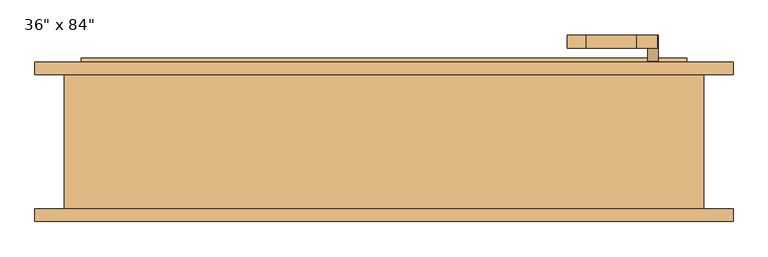
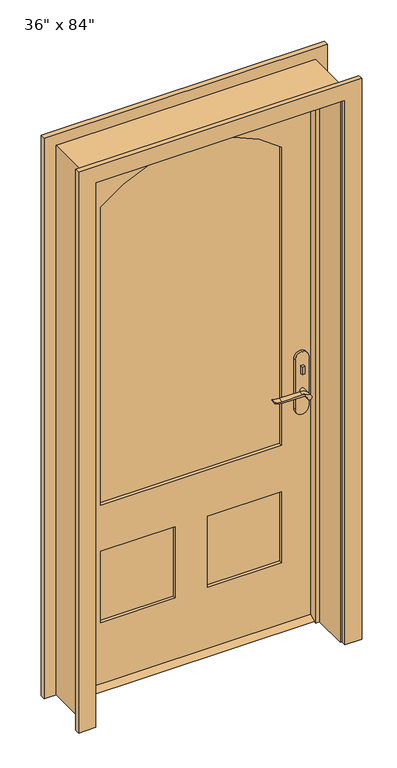
"""IFC4 building model written with IfcOpenShell, lengths in millimetres: door geometry."""

from ifc_helpers import new_model, si_unit, point, frame, frame_2d, origin, place, context, project, spatial, polyline, circle_curve, trimmed, segment, composite_curve, outline, extrude, faceted_brep, source, transform, mapped, element, save


def door_4a215221(model_context):
    return source(origin(), model_context, "Body", "SolidModel", [
        extrude(outline(polyline([(63.5, 12.7), (98.425, 12.7), (123.825, 0.0), (38.1, 0.0), (63.5, 12.7)])), frame((-457.2, 0.0, 0.0), z_axis=(1.0, 0.0, 0.0), x_axis=(0.0, 1.0, 0.0)), (0.0, 0.0, 1.0), 914.4),
        extrude(outline(polyline([(411.4, 43.5), (401.4, 43.5), (401.4, 53.5), (411.4, 53.5), (411.4, 43.5)])), frame((0.0, 0.0, 981.9), z_axis=(0.0, 0.0, 1.0), x_axis=(1.0, 0.0, 0.0)), (0.0, 0.0, 1.0), 30.0),
        extrude(outline(composite_curve([segment(trimmed(circle_curve(frame_2d((996.9, 406.4)), 8.0), [point((996.9, 398.4))], [point((996.9, 414.4))], False, "CARTESIAN"), True, "CONTINUOUS"), segment(trimmed(circle_curve(frame_2d((996.9, 406.4)), 8.0), [point((996.9, 414.4))], [point((996.9, 398.4))], False, "CARTESIAN"), True, "CONTINUOUS")], self_intersect=False)), frame((0.0, 108.425, 0.0), z_axis=(0.0, 1.0, 0.0), x_axis=(0.0, 0.0, 1.0)), (0.0, 0.0, 1.0), 10.0),
        extrude(outline(composite_curve([segment(trimmed(circle_curve(frame_2d((897.1555521, 382.7324871)), 37.2832219), [point((919.0523287, 412.9081363))], [point((934.4, 381.0325667))], False, "CARTESIAN"), True, "CONTINUOUS"), segment(polyline([(934.4, 381.0325667), (934.4, 304.7564091)]), True, "CONTINUOUS"), segment(trimmed(circle_curve(frame_2d((1017.6850638, 304.8227909)), 83.2850902), [point((934.4, 304.7564091))], [point((939.4, 276.4))], True, "CARTESIAN"), True, "CONTINUOUS"), segment(polyline([(939.4, 276.4), (936.6135558, 276.4)]), True, "CONTINUOUS"), segment(trimmed(circle_curve(frame_2d((986.6709207, 308.3396612)), 59.3791355), [point((936.6135558, 276.4))], [point((927.4, 304.7564091))], False, "CARTESIAN"), True, "CONTINUOUS"), segment(polyline([(927.4, 304.7564091), (927.4, 381.0138099)]), True, "CONTINUOUS"), segment(trimmed(circle_curve(frame_2d((909.2738613, 381.0138099)), 18.1261387), [point((927.4, 381.0138099))], [point((914.4, 398.4))], True, "CARTESIAN"), True, "CONTINUOUS"), segment(trimmed(circle_curve(frame_2d((914.4, 406.4)), 8.0), [point((914.4, 398.4))], [point((919.0523287, 412.9081363))], False, "CARTESIAN"), True, "CONTINUOUS")], self_intersect=False)), frame((0.0, 3.5, 0.0), z_axis=(0.0, 1.0, 0.0), x_axis=(0.0, 0.0, 1.0)), (0.0, 0.0, 1.0), 20.0),
        extrude(outline(composite_curve([segment(trimmed(circle_curve(frame_2d((914.4, 406.4)), 8.0), [point((914.3999903, 398.4))], [point((919.0523287, 412.9081363))], False, "CARTESIAN"), True, "CONTINUOUS"), segment(trimmed(circle_curve(frame_2d((897.1555521, 382.7324871)), 37.2832219), [point((919.0523287, 412.9081363))], [point((934.4, 381.0325667))], False, "CARTESIAN"), True, "CONTINUOUS"), segment(polyline([(934.4, 381.0325667), (934.4, 304.7564091)]), True, "CONTINUOUS"), segment(trimmed(circle_curve(frame_2d((1017.6850638, 304.8227909)), 83.2850902), [point((934.4, 304.7564091))], [point((939.4, 276.4))], True, "CARTESIAN"), True, "CONTINUOUS"), segment(polyline([(939.4, 276.4), (936.6135558, 276.4)]), True, "CONTINUOUS"), segment(trimmed(circle_curve(frame_2d((986.6709207, 308.3396612)), 59.3791355), [point((936.6135558, 276.4))], [point((927.4, 304.7564091))], False, "CARTESIAN"), True, "CONTINUOUS"), segment(polyline([(927.4, 304.7564091), (927.4, 381.0138122)]), True, "CONTINUOUS"), segment(trimmed(circle_curve(frame_2d((909.2738682, 381.0138122)), 18.1261318), [point((927.4, 381.0138122))], [point((914.3999903, 398.4))], True, "CARTESIAN"), True, "CONTINUOUS")], self_intersect=False)), frame((0.0, 138.425, 0.0), z_axis=(0.0, 1.0, 0.0), x_axis=(0.0, 0.0, 1.0)), (0.0, 0.0, 1.0), 20.0),
        extrude(outline(composite_curve([segment(trimmed(circle_curve(frame_2d((914.4, 406.4)), 8.0), [point((914.4, 398.4))], [point((914.4, 414.4))], False, "CARTESIAN"), True, "CONTINUOUS"), segment(trimmed(circle_curve(frame_2d((914.4, 406.4)), 8.0), [point((914.4, 414.4))], [point((914.4, 398.4))], False, "CARTESIAN"), True, "CONTINUOUS")], self_intersect=False)), frame((0.0, 23.5, 0.0), z_axis=(0.0, 1.0, 0.0), x_axis=(0.0, 0.0, 1.0)), (0.0, 0.0, 1.0), 30.0),
        extrude(outline(composite_curve([segment(trimmed(circle_curve(frame_2d((914.4, 406.4)), 8.0), [point((914.4, 398.4))], [point((914.4, 414.4))], False, "CARTESIAN"), True, "CONTINUOUS"), segment(trimmed(circle_curve(frame_2d((914.4, 406.4)), 8.0), [point((914.4, 414.4))], [point((914.4, 398.4))], False, "CARTESIAN"), True, "CONTINUOUS")], self_intersect=False)), frame((0.0, 108.425, 0.0), z_axis=(0.0, 1.0, 0.0), x_axis=(0.0, 0.0, 1.0)), (0.0, 0.0, 1.0), 30.0),
        extrude(outline(composite_curve([segment(polyline([(844.4, 431.4), (1039.4, 431.4)]), True, "CONTINUOUS"), segment(trimmed(circle_curve(frame_2d((1039.4, 406.4)), 25.0), [point((1039.4, 431.4))], [point((1039.4, 381.4))], False, "CARTESIAN"), True, "CONTINUOUS"), segment(polyline([(1039.4, 381.4), (844.4, 381.4)]), True, "CONTINUOUS"), segment(trimmed(circle_curve(frame_2d((844.4, 406.4)), 25.0), [point((844.4, 381.4))], [point((844.4, 431.4))], False, "CARTESIAN"), True, "CONTINUOUS")], self_intersect=False)), frame((0.0, 53.5, 0.0), z_axis=(0.0, 1.0, 0.0), x_axis=(0.0, 0.0, 1.0)), (0.0, 0.0, 1.0), 10.0),
        extrude(outline(composite_curve([segment(polyline([(844.4, 431.4), (1039.4, 431.4)]), True, "CONTINUOUS"), segment(trimmed(circle_curve(frame_2d((1039.4, 406.4)), 25.0), [point((1039.4, 431.4))], [point((1039.4, 381.4))], False, "CARTESIAN"), True, "CONTINUOUS"), segment(polyline([(1039.4, 381.4), (844.4, 381.4)]), True, "CONTINUOUS"), segment(trimmed(circle_curve(frame_2d((844.4, 406.4)), 25.0), [point((844.4, 381.4))], [point((844.4, 431.4))], False, "CARTESIAN"), True, "CONTINUOUS")], self_intersect=False)), frame((0.0, 98.425, 0.0), z_axis=(0.0, 1.0, 0.0), x_axis=(0.0, 0.0, 1.0)), (0.0, 0.0, 1.0), 10.0),
        extrude(outline(polyline([(2133.6, -457.2), (12.7, -457.2), (12.7, 457.2), (2133.6, 457.2), (2133.6, -457.2)]), holes=[composite_curve([segment(polyline([(714.375, -336.55), (1885.95, -336.55)]), True, "CONTINUOUS"), segment(trimmed(circle_curve(frame_2d((1503.52125, 0.0)), 509.42875), [point((1885.95, -336.55))], [point((1885.95, 336.55))], True, "CARTESIAN"), True, "CONTINUOUS"), segment(polyline([(1885.95, 336.55), (714.375, 336.55), (714.375, -336.55)]), True, "CONTINUOUS")], self_intersect=False), polyline([(533.4, -60.325), (254.0, -60.325), (254.0, -336.55), (533.4, -336.55), (533.4, -60.325)]), polyline([(533.4, 336.55), (254.0, 336.55), (254.0, 60.325), (533.4, 60.325), (533.4, 336.55)])]), frame((0.0, 63.5, 0.0), z_axis=(0.0, 1.0, 0.0), x_axis=(0.0, 0.0, 1.0)), (0.0, 0.0, 1.0), 34.925),
        faceted_brep([(482.6, 98.425, 0.0), (482.6, -104.775, 0.0), (457.2, -104.775, 0.0), (457.2, 28.575, 0.0), (444.5, 28.575, 0.0), (444.5, 63.5, 0.0), (457.2, 63.5, 0.0), (457.2, 98.425, 0.0), (482.6, 98.425, 2159.0), (482.6, -104.775, 2159.0), (-482.6, -104.775, 2159.0), (-482.6, -104.775, 0.0), (-457.2, -104.775, 0.0), (-457.2, -104.775, 2133.6), (457.2, -104.775, 2133.6), (457.2, 28.575, 2133.6), (-457.2, 28.575, 2133.6), (-457.2, 28.575, 0.0), (-444.5, 28.575, 0.0), (-444.5, 28.575, 2120.9), (444.5, 28.575, 2120.9), (444.5, 63.5, 2120.9), (-444.5, 63.5, 2120.9), (-444.5, 63.5, 0.0), (-457.2, 63.5, 0.0), (-457.2, 63.5, 2133.6), (457.2, 63.5, 2133.6), (457.2, 98.425, 2133.6), (-457.2, 98.425, 2133.6), (-457.2, 98.425, 0.0), (-482.6, 98.425, 0.0), (-482.6, 98.425, 2159.0)], [[[0, 1, 2, 3, 4, 5, 6, 7]], [[1, 0, 8, 9]], [[2, 1, 9, 10, 11, 12, 13, 14]], [[3, 2, 14, 15]], [[4, 3, 15, 16, 17, 18, 19, 20]], [[5, 4, 20, 21]], [[6, 5, 21, 22, 23, 24, 25, 26]], [[7, 6, 26, 27]], [[0, 7, 27, 28, 29, 30, 31, 8]], [[9, 8, 31, 10]], [[15, 14, 13, 16]], [[21, 20, 19, 22]], [[27, 26, 25, 28]], [[30, 29, 24, 23, 18, 17, 12, 11]], [[10, 31, 30, 11]], [[16, 13, 12, 17]], [[22, 19, 18, 23]], [[28, 25, 24, 29]]]),
        extrude(outline(polyline([(-60.325, 75.1416667), (-336.55, 75.1416667), (-336.55, 86.7833333), (-60.325, 86.7833333), (-60.325, 75.1416667)])), frame((0.0, 0.0, 254.0), z_axis=(0.0, 0.0, 1.0), x_axis=(1.0, 0.0, 0.0)), (0.0, 0.0, 1.0), 279.4),
        extrude(outline(polyline([(336.55, 75.1416667), (60.325, 75.1416667), (60.325, 86.7833333), (336.55, 86.7833333), (336.55, 75.1416667)])), frame((0.0, 0.0, 254.0), z_axis=(0.0, 0.0, 1.0), x_axis=(1.0, 0.0, 0.0)), (0.0, 0.0, 1.0), 279.4),
        extrude(outline(composite_curve([segment(polyline([(714.375, -336.55), (714.375, 336.55), (1885.95, 336.55)]), True, "CONTINUOUS"), segment(trimmed(circle_curve(frame_2d((1503.52125, 0.0)), 509.42875), [point((1885.95, 336.55))], [point((1885.95, -336.55))], False, "CARTESIAN"), True, "CONTINUOUS"), segment(polyline([(1885.95, -336.55), (714.375, -336.55)]), True, "CONTINUOUS")], self_intersect=False)), frame((0.0, 77.47, 0.0), z_axis=(0.0, 1.0, 0.0), x_axis=(0.0, 0.0, 1.0)), (0.0, 0.0, 1.0), 6.985),
        extrude(outline(polyline([(0.0, -527.05), (0.0, -463.55), (2139.95, -463.55), (2139.95, 463.55), (0.0, 463.55), (0.0, 527.05), (2203.45, 527.05), (2203.45, -527.05), (0.0, -527.05)])), frame((0.0, -123.825, 0.0), z_axis=(0.0, 1.0, 0.0), x_axis=(0.0, 0.0, 1.0)), (0.0, 0.0, 1.0), 19.05),
        extrude(outline(polyline([(0.0, -527.05), (0.0, -463.55), (2139.95, -463.55), (2139.95, 463.55), (0.0, 463.55), (0.0, 527.05), (2203.45, 527.05), (2203.45, -527.05), (0.0, -527.05)])), frame((0.0, 98.425, 0.0), z_axis=(0.0, 1.0, 0.0), x_axis=(0.0, 0.0, 1.0)), (0.0, 0.0, 1.0), 19.05),
    ])


if __name__ == "__main__":
    model = new_model("IFC4")
    model_context = context("Model", 3, world=origin())
    ifc_project = project(units=[si_unit("LENGTHUNIT", "METRE", prefix="MILLI")], contexts=[model_context])
    site = spatial("IfcSite", under=ifc_project)
    building = spatial("IfcBuilding", under=site)
    placement = place(None, origin())
    door_shape = door_4a215221(model_context)
    element("IfcDoor", 1, ObjectType="36\" x 84\"", at=placement, inside=building, context=model_context, shape_type="MappedRepresentation", body=[
        mapped(door_shape, transform((0.0, 0.0, 0.0), x_axis=(1.0, 0.0, 0.0), y_axis=(0.0, 1.0, 0.0), z_axis=(0.0, 0.0, 1.0))),
    ])
    save(model, "model.ifc")

# Revit data of these elements
# Type "36\" x 84\""
#   Type Mark = "8"
#   Assembly Code = "B2030100"
#   Analytic Construction = "French door, wood frame with single glass"
#   Threshold Offset [instance default] = 0' - 0 1/2"
#   Thickness = 0' - 1 3/8"
#   Thermal Resistance (R) = 1.0696 (h·ft²·°F)/BTU
#   Swing Angle [instance default] = 90.00°
#   Stiles = 0' - 4 3/4"
#   Rough Width = 3' - 2"
#   Rough Height = 7' - 1"
#   Radius = 1' - 8.05625"
#   Lock Rail = 0' - 7 1/8"
#   Height = 7' - 0"
#   Width = 3' - 0"
#   Heat Transfer Coefficient (U) = 0.9350 BTU/(h·ft²·°F)
#   Door Offset [instance default] = 0' - 0"
#   Bottom Rail = 0' - 9 1/2"
#   Threshold [instance default] = yes
#   Function = 1
#   Exterior Trim [instance default] = yes
#   Trim Material = Cherry
#   Threshold Material = Cherry
#   Panel Material = Cherry
#   Glazing = Glass
#   Frame Material = Cherry
#   Door Handle Material = Aluminum
#   Visual Light Transmittance = 0
#   Solar Heat Gain Coefficient = 0
#   Wall Closure = (empty or 0)
#   Construction Type = (empty or 0)
# Element 1 (IfcDoor, "36\" x 84\"")
#   Materials on its faces: "Cherry", "Aluminum", "Glass"
# Materials
#   "Cherry": class "Wood", colour RGB 226 177 128, transparency 0, Description = "Prunus Serotina", Cost = 0
#   "Glass": class "Glass", colour RGB 0 128 192, transparency 0.75, Description = "Soda Lime Glass", Cost = 0
#   "Aluminum": class "Metal", colour RGB 247 247 247, transparency 0, Description = "Aluminum 6061", Cost = 0
